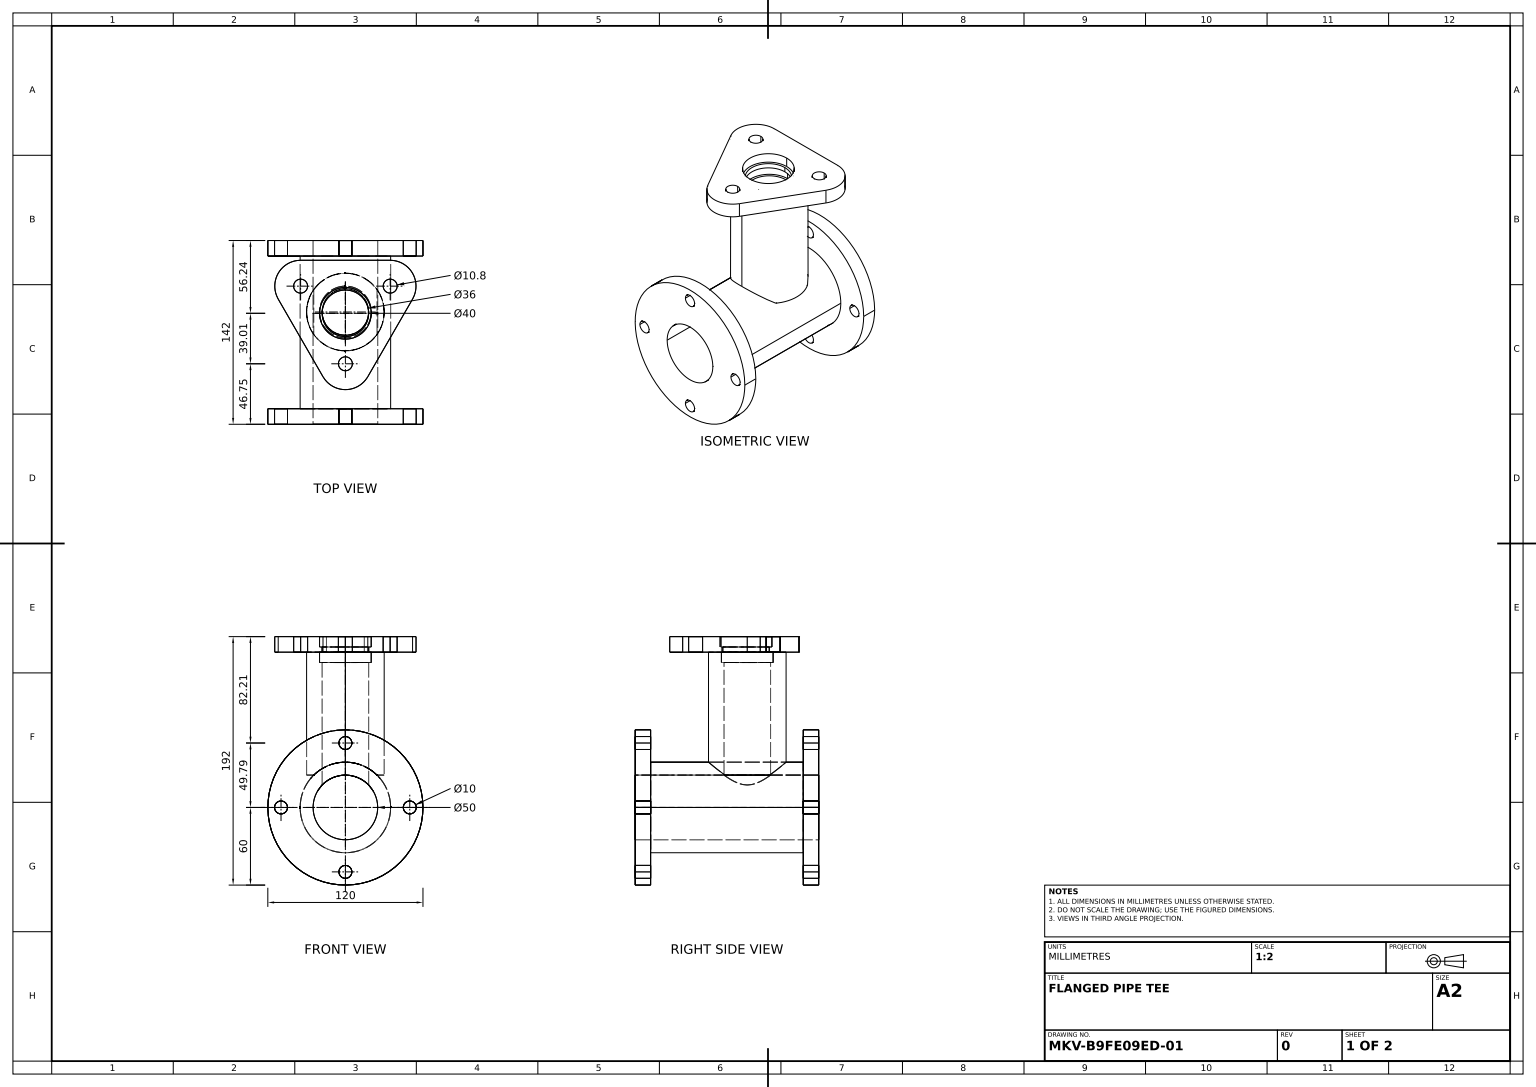
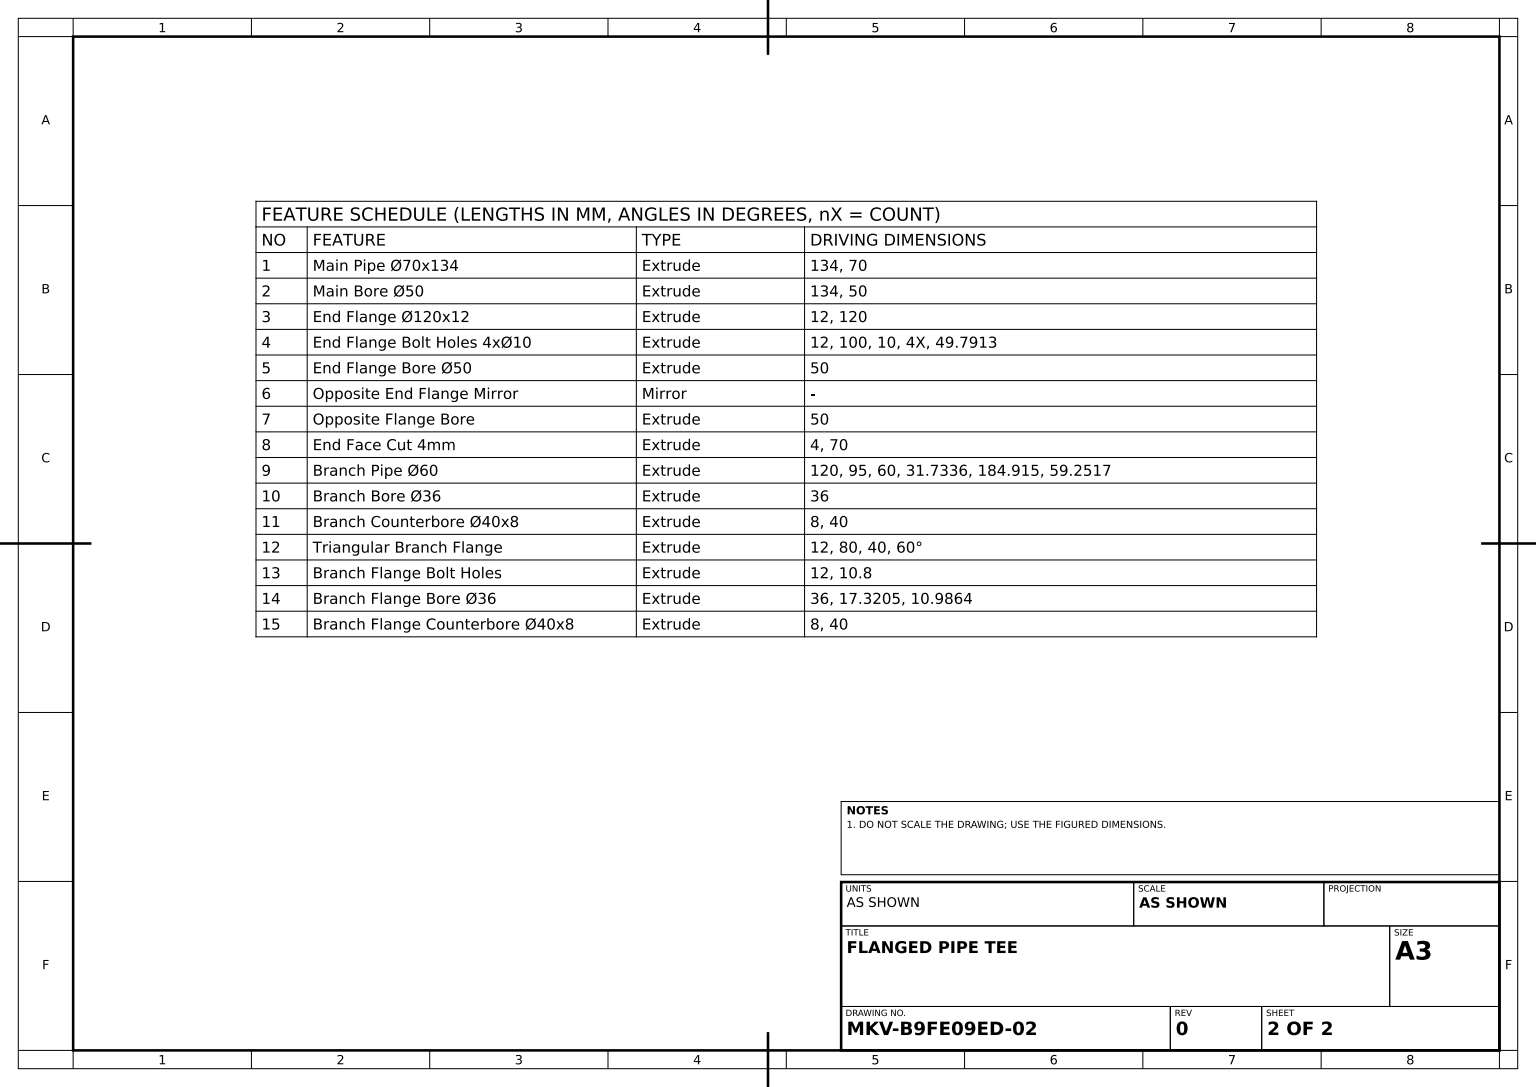
from build123d import *

# Parameters (mm, degrees)
MAIN_PIPE_SKETCH_R                   = 35
MAIN_PIPE_70X134_DEPTH               = 134
MAIN_BORE_SKETCH_R                   = 25
MAIN_BORE_50_DEPTH                   = 134
END_FLANGE_SKETCH_R                  = 60
END_FLANGE_120X12_DEPTH              = 12
END_FLANGE_BOLT_HOLES_SKETCH_R       = 5
END_FLANGE_BOLT_HOLES_4X_10_DEPTH    = 12
END_FLANGE_BORE_SKETCH_R             = 25
END_FLANGE_BORE_50_DEPTH             = 169.866811422
OPPOSITE_FLANGE_BORE_SKETCH_R        = 25
OPPOSITE_FLANGE_BORE_DEPTH           = 166.420675854
END_FACE_CUT_SKETCH_R                = 35
END_FACE_CUT_4MM_DEPTH               = 4
BRANCH_PIPE_SKETCH_R                 = 30
BRANCH_PIPE_60_DEPTH                 = 95
BRANCH_BORE_36_REACH                 = 241.408
BRANCH_BORE_36_END_RADIUS            = 25
BRANCH_BORE_SKETCH_R                 = 18
BRANCH_COUNTERBORE_SKETCH_R          = 20
BRANCH_COUNTERBORE_40X8_DEPTH        = 8
TRIANGULAR_BRANCH_FLANGE_DEPTH       = 12
BRANCH_FLANGE_HOLES_SKETCH_R         = 5.4
BRANCH_FLANGE_BOLT_HOLES_DEPTH       = 12
BRANCH_FLANGE_BORE_36_REACH          = 250.556
BRANCH_FLANGE_BORE_SKETCH_R          = 18
BRANCH_FLANGE_COUNTERBORE_SKETCH_R   = 20
BRANCH_FLANGE_COUNTERBORE_40X8_DEPTH = 8


with BuildPart() as part:
    # Main Pipe Sketch → Main Pipe Ø70x134 (new body)
    with BuildSketch(Plane.XY):
        Circle(MAIN_PIPE_SKETCH_R)
    extrude(amount=MAIN_PIPE_70X134_DEPTH)

    # Main Bore Sketch → Main Bore Ø50 (cut)
    with BuildSketch(Plane.XY.offset(134)):
        Circle(MAIN_BORE_SKETCH_R)
    extrude(amount=-MAIN_BORE_50_DEPTH, mode=Mode.SUBTRACT)

    # End Flange Sketch → End Flange Ø120x12 (add)
    with BuildSketch(Plane.XY.offset(134)):
        Circle(END_FLANGE_SKETCH_R)
    end_flange_120x12 = extrude(amount=END_FLANGE_120X12_DEPTH)

    # End Flange Bolt Holes Sketch → End Flange Bolt Holes 4xØ10 (cut)
    with BuildSketch(Plane.XY.offset(146)):
        with Locations((0, 49.791299633)):
            Circle(END_FLANGE_BOLT_HOLES_SKETCH_R)
        with Locations((49.791299633, 0)):
            Circle(END_FLANGE_BOLT_HOLES_SKETCH_R)
        with Locations((0, -49.791299633)):
            Circle(END_FLANGE_BOLT_HOLES_SKETCH_R)
        with Locations((-49.791299633, 0)):
            Circle(END_FLANGE_BOLT_HOLES_SKETCH_R)
    end_flange_bolt_holes_4x_10 = extrude(amount=-END_FLANGE_BOLT_HOLES_4X_10_DEPTH, mode=Mode.SUBTRACT)

    # End Flange Bore Sketch → End Flange Bore Ø50 (cut, through all)
    with BuildSketch(Plane.XY.offset(146)):
        Circle(END_FLANGE_BORE_SKETCH_R)
    extrude(amount=-END_FLANGE_BORE_50_DEPTH, mode=Mode.SUBTRACT)

    # Opposite End Flange Mirror: End Flange Ø120x12, End Flange Bolt Holes 4xØ10 across plane
    add(end_flange_120x12.mirror(Plane.XY.offset(75)))
    add(end_flange_bolt_holes_4x_10.mirror(Plane.XY.offset(75)), mode=Mode.SUBTRACT)

    # Opposite Flange Bore Sketch → Opposite Flange Bore (cut, through all)
    with BuildSketch(Plane(origin=(0, 0, 4), x_dir=(-1, 0, 0), z_dir=(0, 0, -1))):
        with Locations(Location((0, 0, 0), (0, 0, 180))):
            Circle(OPPOSITE_FLANGE_BORE_SKETCH_R)
    extrude(amount=-OPPOSITE_FLANGE_BORE_DEPTH, mode=Mode.SUBTRACT)

    # End Face Cut Sketch → End Face Cut 4mm (cut)
    with BuildSketch(Plane(origin=(0, 0, 0), x_dir=(-1, 0, 0), z_dir=(0, 0, -1))):
        Circle(END_FACE_CUT_SKETCH_R)
    extrude(amount=-END_FACE_CUT_4MM_DEPTH, mode=Mode.SUBTRACT)

    # Branch Pipe Sketch → Branch Pipe Ø60 (add)
    with BuildSketch(Plane(origin=(0, 120, 0), x_dir=(1, 0, 0), z_dir=(0, 1, 0))):
        with Locations(Location((0, -59.251741082, 0), (0, 0, 270))):
            Circle(BRANCH_PIPE_SKETCH_R)
    extrude(amount=-BRANCH_PIPE_60_DEPTH)

    # Branch Bore Ø36: up to this cylinder (the profile starts outside it)
    branch_bore_36_end = Plane(origin=(0, 0, 59.251741), z_dir=(0, 0, 1)) * Cylinder(BRANCH_BORE_36_END_RADIUS, 533.816, mode=Mode.PRIVATE)
    # Branch Bore Sketch → Branch Bore Ø36 (cut, up to the surface)
    with BuildSketch(Plane(origin=(0, 120, 0), x_dir=(1, 0, 0), z_dir=(0, 1, 0)), mode=Mode.PRIVATE) as branch_bore_36_sk1:
        with Locations(Location((0, -59.251741082, 0), (0, 0, 270))):
            Circle(BRANCH_BORE_SKETCH_R)
    branch_bore_36_tool1 = extrude(branch_bore_36_sk1.sketch, amount=-BRANCH_BORE_36_REACH, mode=Mode.PRIVATE) - branch_bore_36_end
    add(branch_bore_36_tool1.solids().sort_by_distance((0, 120, 59.251741))[0], mode=Mode.SUBTRACT)

    # Branch Counterbore Sketch → Branch Counterbore Ø40x8 (cut)
    with BuildSketch(Plane(origin=(0, 120, 0), x_dir=(1, 0, 0), z_dir=(0, 1, 0))):
        with Locations(Location((0, -59.251741082, 0), (0, 0, 270))):
            Circle(BRANCH_COUNTERBORE_SKETCH_R)
    extrude(amount=-BRANCH_COUNTERBORE_40X8_DEPTH, mode=Mode.SUBTRACT)

    # Branch Flange Sketch → Triangular Branch Flange (add)
    with BuildSketch(Plane(origin=(0, 120, 0), x_dir=(1, 0, 0), z_dir=(0, 1, 0))):
        with BuildLine():
            Line((-51.961524227, -49.251741082), (-17.320508076, -109.251741082))
            ThreePointArc((-17.320508076, -109.251741082), (0, -119.251741082), (17.320508076, -109.251741082))
            Line((17.320508076, -109.251741082), (51.961524227, -49.251741082))
            ThreePointArc((51.961524227, -49.251741082), (51.961524227, -29.251741082), (34.641016151, -19.251741082))
            Line((34.641016151, -19.251741082), (-34.641016151, -19.251741082))
            ThreePointArc((-34.641016151, -19.251741082), (-51.961524227, -29.251741082), (-51.961524227, -49.251741082))
        make_face()
    extrude(amount=TRIANGULAR_BRANCH_FLANGE_DEPTH)

    # Branch Flange Holes Sketch → Branch Flange Bolt Holes (cut)
    with BuildSketch(Plane(origin=(0, 132, 0), x_dir=(1, 0, 0), z_dir=(0, 1, 0))):
        with Locations(Location((-34.641016151, -39.251741082, 0), (0, 0, 270))):
            Circle(BRANCH_FLANGE_HOLES_SKETCH_R)
        with Locations(Location((34.641016151, -39.251741082, 0), (0, 0, 90))):
            Circle(BRANCH_FLANGE_HOLES_SKETCH_R)
        with Locations(Location((0, -99.251741082, 0), (0, 0, 270))):
            Circle(BRANCH_FLANGE_HOLES_SKETCH_R)
    extrude(amount=-BRANCH_FLANGE_BOLT_HOLES_DEPTH, mode=Mode.SUBTRACT)

    # Branch Flange Bore Sketch → Branch Flange Bore Ø36 (cut, up to next)
    with BuildSketch(Plane(origin=(0, 132, 0), x_dir=(1, 0, 0), z_dir=(0, 1, 0)), mode=Mode.PRIVATE) as branch_flange_bore_36_sk1:
        with Locations(Location((0, -60.238145752, 0), (0, 0, 270))):
            Circle(BRANCH_FLANGE_BORE_SKETCH_R)
    branch_flange_bore_36_tool1 = extrude(branch_flange_bore_36_sk1.sketch, amount=-BRANCH_FLANGE_BORE_36_REACH, mode=Mode.PRIVATE) & part.part
    add(branch_flange_bore_36_tool1.solids().sort_by_distance((0, 132, 60.238146))[0], mode=Mode.SUBTRACT)

    # Branch Flange Counterbore Sketch → Branch Flange Counterbore Ø40x8 (cut)
    with BuildSketch(Plane(origin=(0, 132, 0), x_dir=(1, 0, 0), z_dir=(0, 1, 0))):
        with Locations(Location((0, -60.238145752, 0), (0, 0, 270))):
            Circle(BRANCH_FLANGE_COUNTERBORE_SKETCH_R)
    extrude(amount=-BRANCH_FLANGE_COUNTERBORE_40X8_DEPTH, mode=Mode.SUBTRACT)


solid = part.part
